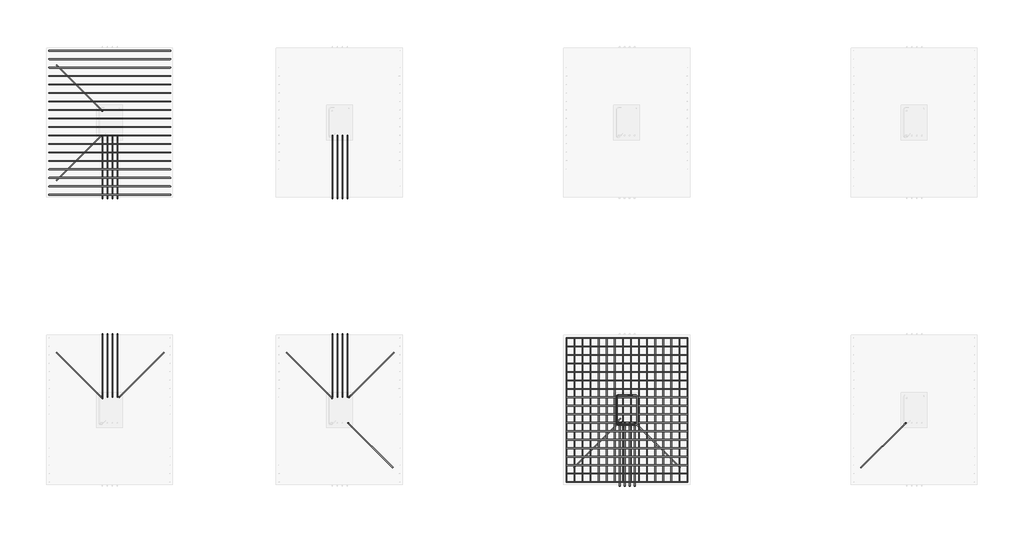
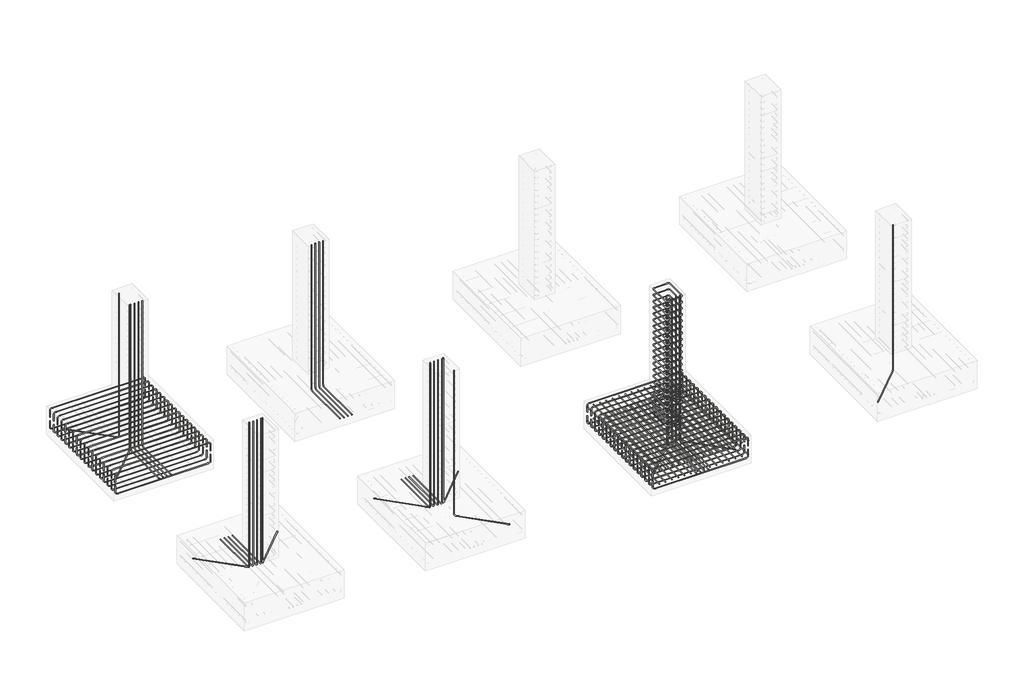
# One storey, part 4 of 33: 22 reinforcing bars.
"""IFC4 building model written with IfcOpenShell, lengths in millimetres."""

from ifc_helpers import new_model, si_unit, point, frame, origin, place, context, project, spatial, polyline, circle_curve, trimmed, segment, composite_curve, source, transform, mapped, element, save
from ifc_brep_helpers import swept_disk

model = new_model("IFC4")

# Units and contexts
model_context = context("Model", 3, world=origin())
ifc_project = project(units=[si_unit("LENGTHUNIT", "METRE", prefix="MILLI")], contexts=[model_context])

# Site, building, storey
site = spatial("IfcSite", under=ifc_project)
building = spatial("IfcBuilding", under=site)
storey = spatial("IfcBuildingStorey", under=building, Elevation=-3000.0)

# Reinforcing bars
placement = place(None, origin())
reinforcing_bar_shape = source(origin(), model_context, "Body", "SolidModel", [
    swept_disk(composite_curve([segment(polyline([(-5693.4642742, -7044.0608134, -3240.0), (-5693.4642742, -7044.0608134, -3092.7)]), True, "CONTINUOUS"), segment(trimmed(circle_curve(frame((-5647.1142742, -7044.0608134, -3092.7), z_axis=(0.0, 1.0, 0.0), x_axis=(-46.349999999999454, 0.0, 0.0)), 46.35), [point((-5693.4642742, -7044.0608134, -3092.7))], [point((-5647.1142742, -7044.0608134, -3046.35))], True, "CARTESIAN"), True, "CONTINUOUS"), segment(polyline([(-5647.1142742, -7044.0608134, -3046.35), (-3632.5142742, -7044.0608134, -3046.35)]), True, "CONTINUOUS"), segment(trimmed(circle_curve(frame((-3632.5142742, -7044.0608134, -3092.7), z_axis=(0.0, 1.0, 0.0), x_axis=(0.0, 0.0, 46.34999999999991)), 46.35), [point((-3632.5142742, -7044.0608134, -3046.35))], [point((-3586.1642742, -7044.0608134, -3092.7))], True, "CARTESIAN"), True, "CONTINUOUS"), segment(polyline([(-3586.1642742, -7044.0608134, -3092.7), (-3586.1642742, -7044.0608134, -3240.0)]), True, "CONTINUOUS")], self_intersect=False), 6.35),
])
element("IfcReinforcingBar", 1, at=placement, inside=storey, context=model_context, shape_type="MappedRepresentation", body=[
    mapped(reinforcing_bar_shape, transform((0.0, 0.0, 0.0), x_axis=(1.0, 0.0, 0.0), y_axis=(0.0, 1.0, 0.0), z_axis=(0.0, 0.0, 1.0))),
    mapped(reinforcing_bar_shape, transform((0.0, -147.4882353, 0.0), x_axis=(1.0, 0.0, 0.0), y_axis=(0.0, 1.0, 0.0), z_axis=(0.0, 0.0, 1.0))),
    mapped(reinforcing_bar_shape, transform((0.0, -294.9764706, 0.0), x_axis=(1.0, 0.0, 0.0), y_axis=(0.0, 1.0, 0.0), z_axis=(0.0, 0.0, 1.0))),
    mapped(reinforcing_bar_shape, transform((0.0, -442.4647059, 0.0), x_axis=(1.0, 0.0, 0.0), y_axis=(0.0, 1.0, 0.0), z_axis=(0.0, 0.0, 1.0))),
    mapped(reinforcing_bar_shape, transform((0.0, -589.9529412, 0.0), x_axis=(1.0, 0.0, 0.0), y_axis=(0.0, 1.0, 0.0), z_axis=(0.0, 0.0, 1.0))),
    mapped(reinforcing_bar_shape, transform((0.0, -737.4411765, 0.0), x_axis=(1.0, 0.0, 0.0), y_axis=(0.0, 1.0, 0.0), z_axis=(0.0, 0.0, 1.0))),
    mapped(reinforcing_bar_shape, transform((0.0, -884.9294118, 0.0), x_axis=(1.0, 0.0, 0.0), y_axis=(0.0, 1.0, 0.0), z_axis=(0.0, 0.0, 1.0))),
    mapped(reinforcing_bar_shape, transform((0.0, -1032.4176471, 0.0), x_axis=(1.0, 0.0, 0.0), y_axis=(0.0, 1.0, 0.0), z_axis=(0.0, 0.0, 1.0))),
    mapped(reinforcing_bar_shape, transform((0.0, -1179.9058824, 0.0), x_axis=(1.0, 0.0, 0.0), y_axis=(0.0, 1.0, 0.0), z_axis=(0.0, 0.0, 1.0))),
    mapped(reinforcing_bar_shape, transform((0.0, -1327.3941176, 0.0), x_axis=(1.0, 0.0, 0.0), y_axis=(0.0, 1.0, 0.0), z_axis=(0.0, 0.0, 1.0))),
    mapped(reinforcing_bar_shape, transform((0.0, -1474.8823529, 0.0), x_axis=(1.0, 0.0, 0.0), y_axis=(0.0, 1.0, 0.0), z_axis=(0.0, 0.0, 1.0))),
    mapped(reinforcing_bar_shape, transform((0.0, -1622.3705882, 0.0), x_axis=(1.0, 0.0, 0.0), y_axis=(0.0, 1.0, 0.0), z_axis=(0.0, 0.0, 1.0))),
    mapped(reinforcing_bar_shape, transform((0.0, -1769.8588235, 0.0), x_axis=(1.0, 0.0, 0.0), y_axis=(0.0, 1.0, 0.0), z_axis=(0.0, 0.0, 1.0))),
    mapped(reinforcing_bar_shape, transform((0.0, -1917.3470588, 0.0), x_axis=(1.0, 0.0, 0.0), y_axis=(0.0, 1.0, 0.0), z_axis=(0.0, 0.0, 1.0))),
    mapped(reinforcing_bar_shape, transform((0.0, -2064.8352941, 0.0), x_axis=(1.0, 0.0, 0.0), y_axis=(0.0, 1.0, 0.0), z_axis=(0.0, 0.0, 1.0))),
    mapped(reinforcing_bar_shape, transform((0.0, -2212.3235294, 0.0), x_axis=(1.0, 0.0, 0.0), y_axis=(0.0, 1.0, 0.0), z_axis=(0.0, 0.0, 1.0))),
    mapped(reinforcing_bar_shape, transform((0.0, -2359.8117647, 0.0), x_axis=(1.0, 0.0, 0.0), y_axis=(0.0, 1.0, 0.0), z_axis=(0.0, 0.0, 1.0))),
    mapped(reinforcing_bar_shape, transform((0.0, -2507.3, 0.0), x_axis=(1.0, 0.0, 0.0), y_axis=(0.0, 1.0, 0.0), z_axis=(0.0, 0.0, 1.0))),
])
reinforcing_bar_2_shape = source(origin(), model_context, "Body", "SolidModel", [
    swept_disk(composite_curve([segment(polyline([(-3586.1642742, -7044.0608134, -3330.080452), (-3586.1642742, -7044.0608134, -3477.380452)]), True, "CONTINUOUS"), segment(trimmed(circle_curve(frame((-3632.5142742, -7044.0608134, -3477.380452), z_axis=(0.0, 1.0, 0.0), x_axis=(46.34999999999991, 0.0, 0.0)), 46.35), [point((-3586.1642742, -7044.0608134, -3477.380452))], [point((-3632.5142742, -7044.0608134, -3523.730452))], True, "CARTESIAN"), True, "CONTINUOUS"), segment(polyline([(-3632.5142742, -7044.0608134, -3523.730452), (-5647.1142742, -7044.0608134, -3523.730452)]), True, "CONTINUOUS"), segment(trimmed(circle_curve(frame((-5647.1142742, -7044.0608134, -3477.380452), z_axis=(0.0, 1.0, 0.0), x_axis=(0.0, 0.0, -46.34999999999991)), 46.35), [point((-5647.1142742, -7044.0608134, -3523.730452))], [point((-5693.4642742, -7044.0608134, -3477.380452))], True, "CARTESIAN"), True, "CONTINUOUS"), segment(polyline([(-5693.4642742, -7044.0608134, -3477.380452), (-5693.4642742, -7044.0608134, -3330.080452)]), True, "CONTINUOUS")], self_intersect=False), 6.35),
])
element("IfcReinforcingBar", 2, at=placement, inside=storey, context=model_context, shape_type="MappedRepresentation", body=[
    mapped(reinforcing_bar_2_shape, transform((0.0, 0.0, 0.0), x_axis=(1.0, 0.0, 0.0), y_axis=(0.0, 1.0, 0.0), z_axis=(0.0, 0.0, 1.0))),
    mapped(reinforcing_bar_2_shape, transform((0.0, -147.4882353, 0.0), x_axis=(1.0, 0.0, 0.0), y_axis=(0.0, 1.0, 0.0), z_axis=(0.0, 0.0, 1.0))),
    mapped(reinforcing_bar_2_shape, transform((0.0, -294.9764706, 0.0), x_axis=(1.0, 0.0, 0.0), y_axis=(0.0, 1.0, 0.0), z_axis=(0.0, 0.0, 1.0))),
    mapped(reinforcing_bar_2_shape, transform((0.0, -442.4647059, 0.0), x_axis=(1.0, 0.0, 0.0), y_axis=(0.0, 1.0, 0.0), z_axis=(0.0, 0.0, 1.0))),
    mapped(reinforcing_bar_2_shape, transform((0.0, -589.9529412, 0.0), x_axis=(1.0, 0.0, 0.0), y_axis=(0.0, 1.0, 0.0), z_axis=(0.0, 0.0, 1.0))),
    mapped(reinforcing_bar_2_shape, transform((0.0, -737.4411765, 0.0), x_axis=(1.0, 0.0, 0.0), y_axis=(0.0, 1.0, 0.0), z_axis=(0.0, 0.0, 1.0))),
    mapped(reinforcing_bar_2_shape, transform((0.0, -884.9294118, 0.0), x_axis=(1.0, 0.0, 0.0), y_axis=(0.0, 1.0, 0.0), z_axis=(0.0, 0.0, 1.0))),
    mapped(reinforcing_bar_2_shape, transform((0.0, -1032.4176471, 0.0), x_axis=(1.0, 0.0, 0.0), y_axis=(0.0, 1.0, 0.0), z_axis=(0.0, 0.0, 1.0))),
    mapped(reinforcing_bar_2_shape, transform((0.0, -1179.9058824, 0.0), x_axis=(1.0, 0.0, 0.0), y_axis=(0.0, 1.0, 0.0), z_axis=(0.0, 0.0, 1.0))),
    mapped(reinforcing_bar_2_shape, transform((0.0, -1327.3941176, 0.0), x_axis=(1.0, 0.0, 0.0), y_axis=(0.0, 1.0, 0.0), z_axis=(0.0, 0.0, 1.0))),
    mapped(reinforcing_bar_2_shape, transform((0.0, -1474.8823529, 0.0), x_axis=(1.0, 0.0, 0.0), y_axis=(0.0, 1.0, 0.0), z_axis=(0.0, 0.0, 1.0))),
    mapped(reinforcing_bar_2_shape, transform((0.0, -1622.3705882, 0.0), x_axis=(1.0, 0.0, 0.0), y_axis=(0.0, 1.0, 0.0), z_axis=(0.0, 0.0, 1.0))),
    mapped(reinforcing_bar_2_shape, transform((0.0, -1769.8588235, 0.0), x_axis=(1.0, 0.0, 0.0), y_axis=(0.0, 1.0, 0.0), z_axis=(0.0, 0.0, 1.0))),
    mapped(reinforcing_bar_2_shape, transform((0.0, -1917.3470588, 0.0), x_axis=(1.0, 0.0, 0.0), y_axis=(0.0, 1.0, 0.0), z_axis=(0.0, 0.0, 1.0))),
    mapped(reinforcing_bar_2_shape, transform((0.0, -2064.8352941, 0.0), x_axis=(1.0, 0.0, 0.0), y_axis=(0.0, 1.0, 0.0), z_axis=(0.0, 0.0, 1.0))),
    mapped(reinforcing_bar_2_shape, transform((0.0, -2212.3235294, 0.0), x_axis=(1.0, 0.0, 0.0), y_axis=(0.0, 1.0, 0.0), z_axis=(0.0, 0.0, 1.0))),
    mapped(reinforcing_bar_2_shape, transform((0.0, -2359.8117647, 0.0), x_axis=(1.0, 0.0, 0.0), y_axis=(0.0, 1.0, 0.0), z_axis=(0.0, 0.0, 1.0))),
    mapped(reinforcing_bar_2_shape, transform((0.0, -2507.3, 0.0), x_axis=(1.0, 0.0, 0.0), y_axis=(0.0, 1.0, 0.0), z_axis=(0.0, 0.0, 1.0))),
])
reinforcing_bar_3_shape = source(origin(), model_context, "Body", "SolidModel", [
    swept_disk(composite_curve([segment(polyline([(-3586.1642742, -9557.7108134, -3447.8614173), (-3586.1642742, -7037.7108134, -3447.8614173)]), True, "CONTINUOUS")], self_intersect=False), 6.35),
])
element("IfcReinforcingBar", 3, at=placement, inside=storey, context=model_context, shape_type="MappedRepresentation", body=[
    mapped(reinforcing_bar_3_shape, transform((0.0, 0.0, 0.0), x_axis=(1.0, 0.0, 0.0), y_axis=(0.0, 1.0, 0.0), z_axis=(0.0, 0.0, 1.0))),
    mapped(reinforcing_bar_3_shape, transform((-140.4866667, 0.0, 0.0), x_axis=(1.0, 0.0, 0.0), y_axis=(0.0, 1.0, 0.0), z_axis=(0.0, 0.0, 1.0))),
    mapped(reinforcing_bar_3_shape, transform((-280.9733333, 0.0, 0.0), x_axis=(1.0, 0.0, 0.0), y_axis=(0.0, 1.0, 0.0), z_axis=(0.0, 0.0, 1.0))),
    mapped(reinforcing_bar_3_shape, transform((-421.46, 0.0, 0.0), x_axis=(1.0, 0.0, 0.0), y_axis=(0.0, 1.0, 0.0), z_axis=(0.0, 0.0, 1.0))),
    mapped(reinforcing_bar_3_shape, transform((-561.9466667, 0.0, 0.0), x_axis=(1.0, 0.0, 0.0), y_axis=(0.0, 1.0, 0.0), z_axis=(0.0, 0.0, 1.0))),
    mapped(reinforcing_bar_3_shape, transform((-702.4333333, 0.0, 0.0), x_axis=(1.0, 0.0, 0.0), y_axis=(0.0, 1.0, 0.0), z_axis=(0.0, 0.0, 1.0))),
    mapped(reinforcing_bar_3_shape, transform((-842.92, 0.0, 0.0), x_axis=(1.0, 0.0, 0.0), y_axis=(0.0, 1.0, 0.0), z_axis=(0.0, 0.0, 1.0))),
    mapped(reinforcing_bar_3_shape, transform((-983.4066667, 0.0, 0.0), x_axis=(1.0, 0.0, 0.0), y_axis=(0.0, 1.0, 0.0), z_axis=(0.0, 0.0, 1.0))),
    mapped(reinforcing_bar_3_shape, transform((-1123.8933333, 0.0, 0.0), x_axis=(1.0, 0.0, 0.0), y_axis=(0.0, 1.0, 0.0), z_axis=(0.0, 0.0, 1.0))),
    mapped(reinforcing_bar_3_shape, transform((-1264.38, 0.0, 0.0), x_axis=(1.0, 0.0, 0.0), y_axis=(0.0, 1.0, 0.0), z_axis=(0.0, 0.0, 1.0))),
    mapped(reinforcing_bar_3_shape, transform((-1404.8666667, 0.0, 0.0), x_axis=(1.0, 0.0, 0.0), y_axis=(0.0, 1.0, 0.0), z_axis=(0.0, 0.0, 1.0))),
    mapped(reinforcing_bar_3_shape, transform((-1545.3533333, 0.0, 0.0), x_axis=(1.0, 0.0, 0.0), y_axis=(0.0, 1.0, 0.0), z_axis=(0.0, 0.0, 1.0))),
    mapped(reinforcing_bar_3_shape, transform((-1685.84, 0.0, 0.0), x_axis=(1.0, 0.0, 0.0), y_axis=(0.0, 1.0, 0.0), z_axis=(0.0, 0.0, 1.0))),
    mapped(reinforcing_bar_3_shape, transform((-1826.3266667, 0.0, 0.0), x_axis=(1.0, 0.0, 0.0), y_axis=(0.0, 1.0, 0.0), z_axis=(0.0, 0.0, 1.0))),
    mapped(reinforcing_bar_3_shape, transform((-1966.8133333, 0.0, 0.0), x_axis=(1.0, 0.0, 0.0), y_axis=(0.0, 1.0, 0.0), z_axis=(0.0, 0.0, 1.0))),
    mapped(reinforcing_bar_3_shape, transform((-2107.3, 0.0, 0.0), x_axis=(1.0, 0.0, 0.0), y_axis=(0.0, 1.0, 0.0), z_axis=(0.0, 0.0, 1.0))),
])
reinforcing_bar_4_shape = source(origin(), model_context, "Body", "SolidModel", [
    swept_disk(composite_curve([segment(polyline([(-5693.4642742, -9557.7108134, -3122.7084113), (-5693.4642742, -7037.7108134, -3122.7084113)]), True, "CONTINUOUS")], self_intersect=False), 6.35),
])
element("IfcReinforcingBar", 4, at=placement, inside=storey, context=model_context, shape_type="MappedRepresentation", body=[
    mapped(reinforcing_bar_4_shape, transform((0.0, 0.0, 0.0), x_axis=(1.0, 0.0, 0.0), y_axis=(0.0, 1.0, 0.0), z_axis=(0.0, 0.0, 1.0))),
    mapped(reinforcing_bar_4_shape, transform((140.4866667, 0.0, 0.0), x_axis=(1.0, 0.0, 0.0), y_axis=(0.0, 1.0, 0.0), z_axis=(0.0, 0.0, 1.0))),
    mapped(reinforcing_bar_4_shape, transform((280.9733333, 0.0, 0.0), x_axis=(1.0, 0.0, 0.0), y_axis=(0.0, 1.0, 0.0), z_axis=(0.0, 0.0, 1.0))),
    mapped(reinforcing_bar_4_shape, transform((421.46, 0.0, 0.0), x_axis=(1.0, 0.0, 0.0), y_axis=(0.0, 1.0, 0.0), z_axis=(0.0, 0.0, 1.0))),
    mapped(reinforcing_bar_4_shape, transform((561.9466667, 0.0, 0.0), x_axis=(1.0, 0.0, 0.0), y_axis=(0.0, 1.0, 0.0), z_axis=(0.0, 0.0, 1.0))),
    mapped(reinforcing_bar_4_shape, transform((702.4333333, 0.0, 0.0), x_axis=(1.0, 0.0, 0.0), y_axis=(0.0, 1.0, 0.0), z_axis=(0.0, 0.0, 1.0))),
    mapped(reinforcing_bar_4_shape, transform((842.92, 0.0, 0.0), x_axis=(1.0, 0.0, 0.0), y_axis=(0.0, 1.0, 0.0), z_axis=(0.0, 0.0, 1.0))),
    mapped(reinforcing_bar_4_shape, transform((983.4066667, 0.0, 0.0), x_axis=(1.0, 0.0, 0.0), y_axis=(0.0, 1.0, 0.0), z_axis=(0.0, 0.0, 1.0))),
    mapped(reinforcing_bar_4_shape, transform((1123.8933333, 0.0, 0.0), x_axis=(1.0, 0.0, 0.0), y_axis=(0.0, 1.0, 0.0), z_axis=(0.0, 0.0, 1.0))),
    mapped(reinforcing_bar_4_shape, transform((1264.38, 0.0, 0.0), x_axis=(1.0, 0.0, 0.0), y_axis=(0.0, 1.0, 0.0), z_axis=(0.0, 0.0, 1.0))),
    mapped(reinforcing_bar_4_shape, transform((1404.8666667, 0.0, 0.0), x_axis=(1.0, 0.0, 0.0), y_axis=(0.0, 1.0, 0.0), z_axis=(0.0, 0.0, 1.0))),
    mapped(reinforcing_bar_4_shape, transform((1545.3533333, 0.0, 0.0), x_axis=(1.0, 0.0, 0.0), y_axis=(0.0, 1.0, 0.0), z_axis=(0.0, 0.0, 1.0))),
    mapped(reinforcing_bar_4_shape, transform((1685.84, 0.0, 0.0), x_axis=(1.0, 0.0, 0.0), y_axis=(0.0, 1.0, 0.0), z_axis=(0.0, 0.0, 1.0))),
    mapped(reinforcing_bar_4_shape, transform((1826.3266667, 0.0, 0.0), x_axis=(1.0, 0.0, 0.0), y_axis=(0.0, 1.0, 0.0), z_axis=(0.0, 0.0, 1.0))),
    mapped(reinforcing_bar_4_shape, transform((1966.8133333, 0.0, 0.0), x_axis=(1.0, 0.0, 0.0), y_axis=(0.0, 1.0, 0.0), z_axis=(0.0, 0.0, 1.0))),
    mapped(reinforcing_bar_4_shape, transform((2107.3, 0.0, 0.0), x_axis=(1.0, 0.0, 0.0), y_axis=(0.0, 1.0, 0.0), z_axis=(0.0, 0.0, 1.0))),
])
reinforcing_bar_5_shape = source(origin(), model_context, "Body", "SolidModel", [
    swept_disk(composite_curve([segment(polyline([(-14693.4642742, -2044.0608134, -3240.0), (-14693.4642742, -2044.0608134, -3092.7)]), True, "CONTINUOUS"), segment(trimmed(circle_curve(frame((-14647.1142742, -2044.0608134, -3092.7), z_axis=(0.0, 1.0, 0.0), x_axis=(-46.350000000000364, 0.0, 0.0)), 46.35), [point((-14693.4642742, -2044.0608134, -3092.7))], [point((-14647.1142742, -2044.0608134, -3046.35))], True, "CARTESIAN"), True, "CONTINUOUS"), segment(polyline([(-14647.1142742, -2044.0608134, -3046.35), (-12632.5142742, -2044.0608134, -3046.35)]), True, "CONTINUOUS"), segment(trimmed(circle_curve(frame((-12632.5142742, -2044.0608134, -3092.7), z_axis=(0.0, 1.0, 0.0), x_axis=(0.0, 0.0, 46.34999999999991)), 46.35), [point((-12632.5142742, -2044.0608134, -3046.35))], [point((-12586.1642742, -2044.0608134, -3092.7))], True, "CARTESIAN"), True, "CONTINUOUS"), segment(polyline([(-12586.1642742, -2044.0608134, -3092.7), (-12586.1642742, -2044.0608134, -3240.0)]), True, "CONTINUOUS")], self_intersect=False), 6.35),
])
element("IfcReinforcingBar", 5, at=placement, inside=storey, context=model_context, shape_type="MappedRepresentation", body=[
    mapped(reinforcing_bar_5_shape, transform((0.0, 0.0, 0.0), x_axis=(1.0, 0.0, 0.0), y_axis=(0.0, 1.0, 0.0), z_axis=(0.0, 0.0, 1.0))),
    mapped(reinforcing_bar_5_shape, transform((0.0, -147.4882353, 0.0), x_axis=(1.0, 0.0, 0.0), y_axis=(0.0, 1.0, 0.0), z_axis=(0.0, 0.0, 1.0))),
    mapped(reinforcing_bar_5_shape, transform((0.0, -294.9764706, 0.0), x_axis=(1.0, 0.0, 0.0), y_axis=(0.0, 1.0, 0.0), z_axis=(0.0, 0.0, 1.0))),
    mapped(reinforcing_bar_5_shape, transform((0.0, -442.4647059, 0.0), x_axis=(1.0, 0.0, 0.0), y_axis=(0.0, 1.0, 0.0), z_axis=(0.0, 0.0, 1.0))),
    mapped(reinforcing_bar_5_shape, transform((0.0, -589.9529412, 0.0), x_axis=(1.0, 0.0, 0.0), y_axis=(0.0, 1.0, 0.0), z_axis=(0.0, 0.0, 1.0))),
    mapped(reinforcing_bar_5_shape, transform((0.0, -737.4411765, 0.0), x_axis=(1.0, 0.0, 0.0), y_axis=(0.0, 1.0, 0.0), z_axis=(0.0, 0.0, 1.0))),
    mapped(reinforcing_bar_5_shape, transform((0.0, -884.9294118, 0.0), x_axis=(1.0, 0.0, 0.0), y_axis=(0.0, 1.0, 0.0), z_axis=(0.0, 0.0, 1.0))),
    mapped(reinforcing_bar_5_shape, transform((0.0, -1032.4176471, 0.0), x_axis=(1.0, 0.0, 0.0), y_axis=(0.0, 1.0, 0.0), z_axis=(0.0, 0.0, 1.0))),
    mapped(reinforcing_bar_5_shape, transform((0.0, -1179.9058824, 0.0), x_axis=(1.0, 0.0, 0.0), y_axis=(0.0, 1.0, 0.0), z_axis=(0.0, 0.0, 1.0))),
    mapped(reinforcing_bar_5_shape, transform((0.0, -1327.3941176, 0.0), x_axis=(1.0, 0.0, 0.0), y_axis=(0.0, 1.0, 0.0), z_axis=(0.0, 0.0, 1.0))),
    mapped(reinforcing_bar_5_shape, transform((0.0, -1474.8823529, 0.0), x_axis=(1.0, 0.0, 0.0), y_axis=(0.0, 1.0, 0.0), z_axis=(0.0, 0.0, 1.0))),
    mapped(reinforcing_bar_5_shape, transform((0.0, -1622.3705882, 0.0), x_axis=(1.0, 0.0, 0.0), y_axis=(0.0, 1.0, 0.0), z_axis=(0.0, 0.0, 1.0))),
    mapped(reinforcing_bar_5_shape, transform((0.0, -1769.8588235, 0.0), x_axis=(1.0, 0.0, 0.0), y_axis=(0.0, 1.0, 0.0), z_axis=(0.0, 0.0, 1.0))),
    mapped(reinforcing_bar_5_shape, transform((0.0, -1917.3470588, 0.0), x_axis=(1.0, 0.0, 0.0), y_axis=(0.0, 1.0, 0.0), z_axis=(0.0, 0.0, 1.0))),
    mapped(reinforcing_bar_5_shape, transform((0.0, -2064.8352941, 0.0), x_axis=(1.0, 0.0, 0.0), y_axis=(0.0, 1.0, 0.0), z_axis=(0.0, 0.0, 1.0))),
    mapped(reinforcing_bar_5_shape, transform((0.0, -2212.3235294, 0.0), x_axis=(1.0, 0.0, 0.0), y_axis=(0.0, 1.0, 0.0), z_axis=(0.0, 0.0, 1.0))),
    mapped(reinforcing_bar_5_shape, transform((0.0, -2359.8117647, 0.0), x_axis=(1.0, 0.0, 0.0), y_axis=(0.0, 1.0, 0.0), z_axis=(0.0, 0.0, 1.0))),
    mapped(reinforcing_bar_5_shape, transform((0.0, -2507.3, 0.0), x_axis=(1.0, 0.0, 0.0), y_axis=(0.0, 1.0, 0.0), z_axis=(0.0, 0.0, 1.0))),
])
reinforcing_bar_6_shape = source(origin(), model_context, "Body", "SolidModel", [
    swept_disk(composite_curve([segment(polyline([(-12586.1642742, -2044.0608134, -3330.080452), (-12586.1642742, -2044.0608134, -3477.380452)]), True, "CONTINUOUS"), segment(trimmed(circle_curve(frame((-12632.5142742, -2044.0608134, -3477.380452), z_axis=(0.0, 1.0, 0.0), x_axis=(46.350000000000364, 0.0, 0.0)), 46.35), [point((-12586.1642742, -2044.0608134, -3477.380452))], [point((-12632.5142742, -2044.0608134, -3523.730452))], True, "CARTESIAN"), True, "CONTINUOUS"), segment(polyline([(-12632.5142742, -2044.0608134, -3523.730452), (-14647.1142742, -2044.0608134, -3523.730452)]), True, "CONTINUOUS"), segment(trimmed(circle_curve(frame((-14647.1142742, -2044.0608134, -3477.380452), z_axis=(0.0, 1.0, 0.0), x_axis=(0.0, 0.0, -46.34999999999991)), 46.35), [point((-14647.1142742, -2044.0608134, -3523.730452))], [point((-14693.4642742, -2044.0608134, -3477.380452))], True, "CARTESIAN"), True, "CONTINUOUS"), segment(polyline([(-14693.4642742, -2044.0608134, -3477.380452), (-14693.4642742, -2044.0608134, -3330.080452)]), True, "CONTINUOUS")], self_intersect=False), 6.35),
])
element("IfcReinforcingBar", 6, at=placement, inside=storey, context=model_context, shape_type="MappedRepresentation", body=[
    mapped(reinforcing_bar_6_shape, transform((0.0, 0.0, 0.0), x_axis=(1.0, 0.0, 0.0), y_axis=(0.0, 1.0, 0.0), z_axis=(0.0, 0.0, 1.0))),
    mapped(reinforcing_bar_6_shape, transform((0.0, -147.4882353, 0.0), x_axis=(1.0, 0.0, 0.0), y_axis=(0.0, 1.0, 0.0), z_axis=(0.0, 0.0, 1.0))),
    mapped(reinforcing_bar_6_shape, transform((0.0, -294.9764706, 0.0), x_axis=(1.0, 0.0, 0.0), y_axis=(0.0, 1.0, 0.0), z_axis=(0.0, 0.0, 1.0))),
    mapped(reinforcing_bar_6_shape, transform((0.0, -442.4647059, 0.0), x_axis=(1.0, 0.0, 0.0), y_axis=(0.0, 1.0, 0.0), z_axis=(0.0, 0.0, 1.0))),
    mapped(reinforcing_bar_6_shape, transform((0.0, -589.9529412, 0.0), x_axis=(1.0, 0.0, 0.0), y_axis=(0.0, 1.0, 0.0), z_axis=(0.0, 0.0, 1.0))),
    mapped(reinforcing_bar_6_shape, transform((0.0, -737.4411765, 0.0), x_axis=(1.0, 0.0, 0.0), y_axis=(0.0, 1.0, 0.0), z_axis=(0.0, 0.0, 1.0))),
    mapped(reinforcing_bar_6_shape, transform((0.0, -884.9294118, 0.0), x_axis=(1.0, 0.0, 0.0), y_axis=(0.0, 1.0, 0.0), z_axis=(0.0, 0.0, 1.0))),
    mapped(reinforcing_bar_6_shape, transform((0.0, -1032.4176471, 0.0), x_axis=(1.0, 0.0, 0.0), y_axis=(0.0, 1.0, 0.0), z_axis=(0.0, 0.0, 1.0))),
    mapped(reinforcing_bar_6_shape, transform((0.0, -1179.9058824, 0.0), x_axis=(1.0, 0.0, 0.0), y_axis=(0.0, 1.0, 0.0), z_axis=(0.0, 0.0, 1.0))),
    mapped(reinforcing_bar_6_shape, transform((0.0, -1327.3941176, 0.0), x_axis=(1.0, 0.0, 0.0), y_axis=(0.0, 1.0, 0.0), z_axis=(0.0, 0.0, 1.0))),
    mapped(reinforcing_bar_6_shape, transform((0.0, -1474.8823529, 0.0), x_axis=(1.0, 0.0, 0.0), y_axis=(0.0, 1.0, 0.0), z_axis=(0.0, 0.0, 1.0))),
    mapped(reinforcing_bar_6_shape, transform((0.0, -1622.3705882, 0.0), x_axis=(1.0, 0.0, 0.0), y_axis=(0.0, 1.0, 0.0), z_axis=(0.0, 0.0, 1.0))),
    mapped(reinforcing_bar_6_shape, transform((0.0, -1769.8588235, 0.0), x_axis=(1.0, 0.0, 0.0), y_axis=(0.0, 1.0, 0.0), z_axis=(0.0, 0.0, 1.0))),
    mapped(reinforcing_bar_6_shape, transform((0.0, -1917.3470588, 0.0), x_axis=(1.0, 0.0, 0.0), y_axis=(0.0, 1.0, 0.0), z_axis=(0.0, 0.0, 1.0))),
    mapped(reinforcing_bar_6_shape, transform((0.0, -2064.8352941, 0.0), x_axis=(1.0, 0.0, 0.0), y_axis=(0.0, 1.0, 0.0), z_axis=(0.0, 0.0, 1.0))),
    mapped(reinforcing_bar_6_shape, transform((0.0, -2212.3235294, 0.0), x_axis=(1.0, 0.0, 0.0), y_axis=(0.0, 1.0, 0.0), z_axis=(0.0, 0.0, 1.0))),
    mapped(reinforcing_bar_6_shape, transform((0.0, -2359.8117647, 0.0), x_axis=(1.0, 0.0, 0.0), y_axis=(0.0, 1.0, 0.0), z_axis=(0.0, 0.0, 1.0))),
    mapped(reinforcing_bar_6_shape, transform((0.0, -2507.3, 0.0), x_axis=(1.0, 0.0, 0.0), y_axis=(0.0, 1.0, 0.0), z_axis=(0.0, 0.0, 1.0))),
])
element("IfcReinforcingBar", 7, at=placement, inside=storey, context=model_context, shape_type="SolidModel", body=[
    swept_disk(composite_curve([segment(polyline([(-13786.7956786, -3521.6339414, -40.0), (-13786.7956786, -3521.6339414, -3393.65)]), True, "CONTINUOUS"), segment(trimmed(circle_curve(frame((-13819.5700779, -3554.4083407, -3393.65), z_axis=(-0.7071067811865446, 0.7071067811865505, 0.0), x_axis=(32.77439930000037, 32.774399299999914, 0.0)), 46.35), [point((-13786.7956786, -3521.6339414, -3393.65))], [point((-13819.5700779, -3554.4083407, -3440.0))], True, "CARTESIAN"), True, "CONTINUOUS"), segment(polyline([(-13819.5700779, -3554.4083407, -3440.0), (-14564.6131379, -4299.4514007, -3440.0)]), True, "CONTINUOUS")], self_intersect=False), 6.35),
])
element("IfcReinforcingBar", 8, at=placement, inside=storey, context=model_context, shape_type="SolidModel", body=[
    swept_disk(composite_curve([segment(polyline([(-13768.8975726, -3091.6857913, -40.0), (-13768.8975726, -3091.6857913, -3361.434517)]), True, "CONTINUOUS"), segment(trimmed(circle_curve(frame((-13801.6719719, -3058.911392, -3361.434517), z_axis=(0.7071067811865539, 0.7071067811865411, 0.0), x_axis=(32.77439929999855, -32.774399299999914, 0.0)), 46.35), [point((-13768.8975726, -3091.6857913, -3361.434517))], [point((-13801.6719719, -3058.911392, -3407.784517))], True, "CARTESIAN"), True, "CONTINUOUS"), segment(polyline([(-13801.6719719, -3058.911392, -3407.784517), (-14564.6131379, -2295.970226, -3407.784517)]), True, "CONTINUOUS")], self_intersect=False), 6.35),
])
reinforcing_bar_7_shape = source(origin(), model_context, "Body", "SolidModel", [
    swept_disk(composite_curve([segment(polyline([(-13763.8841678, -3523.4938134, -40.0), (-13763.8841678, -3523.4938134, -3393.65)]), True, "CONTINUOUS"), segment(trimmed(circle_curve(frame((-13763.8841678, -3569.8438134, -3393.65), z_axis=(-1.0, 0.0, 0.0), x_axis=(0.0, 46.34999999999991, 0.0)), 46.35), [point((-13763.8841678, -3523.4938134, -3393.65))], [point((-13763.8841678, -3569.8438134, -3440.0))], True, "CARTESIAN"), True, "CONTINUOUS"), segment(polyline([(-13763.8841678, -3569.8438134, -3440.0), (-13763.8841678, -4623.4938134, -3440.0)]), True, "CONTINUOUS")], self_intersect=False), 6.35),
])
element("IfcReinforcingBar", 9, at=placement, inside=storey, context=model_context, shape_type="MappedRepresentation", body=[
    mapped(reinforcing_bar_7_shape, transform((0.0, 0.0, 0.0), x_axis=(1.0, 0.0, 0.0), y_axis=(0.0, 1.0, 0.0), z_axis=(0.0, 0.0, 1.0))),
    mapped(reinforcing_bar_7_shape, transform((86.8979716, 0.0, 0.0), x_axis=(1.0, 0.0, 0.0), y_axis=(0.0, 1.0, 0.0), z_axis=(0.0, 0.0, 1.0))),
    mapped(reinforcing_bar_7_shape, transform((173.7959432, 0.0, 0.0), x_axis=(1.0, 0.0, 0.0), y_axis=(0.0, 1.0, 0.0), z_axis=(0.0, 0.0, 1.0))),
    mapped(reinforcing_bar_7_shape, transform((260.6939148, 0.0, 0.0), x_axis=(1.0, 0.0, 0.0), y_axis=(0.0, 1.0, 0.0), z_axis=(0.0, 0.0, 1.0))),
])
element("IfcReinforcingBar", 10, at=placement, inside=storey, context=model_context, shape_type="SolidModel", body=[
    swept_disk(composite_curve([segment(polyline([(-13768.8975726, -8091.6857913, -40.0), (-13768.8975726, -8091.6857913, -3361.434517)]), True, "CONTINUOUS"), segment(trimmed(circle_curve(frame((-13801.6719719, -8058.911392, -3361.434517), z_axis=(0.7071067811865539, 0.7071067811865411, 0.0), x_axis=(32.77439929999855, -32.77439930000037, 0.0)), 46.35), [point((-13768.8975726, -8091.6857913, -3361.434517))], [point((-13801.6719719, -8058.911392, -3407.784517))], True, "CARTESIAN"), True, "CONTINUOUS"), segment(polyline([(-13801.6719719, -8058.911392, -3407.784517), (-14564.6131379, -7295.970226, -3407.784517)]), True, "CONTINUOUS")], self_intersect=False), 6.35),
])
element("IfcReinforcingBar", 11, at=placement, inside=storey, context=model_context, shape_type="SolidModel", body=[
    swept_disk(composite_curve([segment(polyline([(-13474.2315783, -8073.7876853, -30.2564663), (-13474.2315783, -8073.7876853, -3383.9064663)]), True, "CONTINUOUS"), segment(trimmed(circle_curve(frame((-13441.457179, -8041.013286, -3383.9064663), z_axis=(0.7071067811865493, -0.7071067811865459, 0.0), x_axis=(-32.77439929999855, -32.77439929999946, 0.0)), 46.35), [point((-13474.2315783, -8073.7876853, -3383.9064663))], [point((-13441.457179, -8041.013286, -3430.2564663))], True, "CARTESIAN"), True, "CONTINUOUS"), segment(polyline([(-13441.457179, -8041.013286, -3430.2564663), (-12696.414119, -7295.970226, -3430.2564663)]), True, "CONTINUOUS")], self_intersect=False), 6.35),
])
reinforcing_bar_8_shape = source(origin(), model_context, "Body", "SolidModel", [
    swept_disk(composite_curve([segment(polyline([(-13763.8841678, -8071.9278134, -40.0), (-13763.8841678, -8071.9278134, -3393.65)]), True, "CONTINUOUS"), segment(trimmed(circle_curve(frame((-13763.8841678, -8025.5778134, -3393.65), z_axis=(1.0, 0.0, 0.0), x_axis=(0.0, -46.349999999999454, 0.0)), 46.35), [point((-13763.8841678, -8071.9278134, -3393.65))], [point((-13763.8841678, -8025.5778134, -3440.0))], True, "CARTESIAN"), True, "CONTINUOUS"), segment(polyline([(-13763.8841678, -8025.5778134, -3440.0), (-13763.8841678, -6971.9278134, -3440.0)]), True, "CONTINUOUS")], self_intersect=False), 6.35),
])
element("IfcReinforcingBar", 12, at=placement, inside=storey, context=model_context, shape_type="MappedRepresentation", body=[
    mapped(reinforcing_bar_8_shape, transform((0.0, 0.0, 0.0), x_axis=(1.0, 0.0, 0.0), y_axis=(0.0, 1.0, 0.0), z_axis=(0.0, 0.0, 1.0))),
    mapped(reinforcing_bar_8_shape, transform((86.8979716, 0.0, 0.0), x_axis=(1.0, 0.0, 0.0), y_axis=(0.0, 1.0, 0.0), z_axis=(0.0, 0.0, 1.0))),
    mapped(reinforcing_bar_8_shape, transform((173.7959432, 0.0, 0.0), x_axis=(1.0, 0.0, 0.0), y_axis=(0.0, 1.0, 0.0), z_axis=(0.0, 0.0, 1.0))),
    mapped(reinforcing_bar_8_shape, transform((260.6939148, 0.0, 0.0), x_axis=(1.0, 0.0, 0.0), y_axis=(0.0, 1.0, 0.0), z_axis=(0.0, 0.0, 1.0))),
])
element("IfcReinforcingBar", 13, at=placement, inside=storey, context=model_context, shape_type="SolidModel", body=[
    swept_disk(composite_curve([segment(polyline([(-9768.8975726, -8091.6857913, -40.0), (-9768.8975726, -8091.6857913, -3361.434517)]), True, "CONTINUOUS"), segment(trimmed(circle_curve(frame((-9801.6719719, -8058.911392, -3361.434517), z_axis=(0.7071067811865539, 0.7071067811865411, 0.0), x_axis=(32.77439929999855, -32.77439930000037, 0.0)), 46.35), [point((-9768.8975726, -8091.6857913, -3361.434517))], [point((-9801.6719719, -8058.911392, -3407.784517))], True, "CARTESIAN"), True, "CONTINUOUS"), segment(polyline([(-9801.6719719, -8058.911392, -3407.784517), (-10564.6131379, -7295.970226, -3407.784517)]), True, "CONTINUOUS")], self_intersect=False), 6.35),
])
element("IfcReinforcingBar", 14, at=placement, inside=storey, context=model_context, shape_type="SolidModel", body=[
    swept_disk(composite_curve([segment(polyline([(-9492.8328699, -8521.6339414, -40.0), (-9492.8328699, -8521.6339414, -3393.65)]), True, "CONTINUOUS"), segment(trimmed(circle_curve(frame((-9460.0584706, -8554.4083407, -3393.65), z_axis=(-0.7071067811865493, -0.7071067811865459, 0.0), x_axis=(-32.77439929999855, 32.77439930000037, 0.0)), 46.35), [point((-9492.8328699, -8521.6339414, -3393.65))], [point((-9460.0584706, -8554.4083407, -3440.0))], True, "CARTESIAN"), True, "CONTINUOUS"), segment(polyline([(-9460.0584706, -8554.4083407, -3440.0), (-8715.0154106, -9299.4514007, -3440.0)]), True, "CONTINUOUS")], self_intersect=False), 6.35),
])
element("IfcReinforcingBar", 15, at=placement, inside=storey, context=model_context, shape_type="SolidModel", body=[
    swept_disk(composite_curve([segment(polyline([(-9474.2315783, -8073.7876853, -30.2564663), (-9474.2315783, -8073.7876853, -3383.9064663)]), True, "CONTINUOUS"), segment(trimmed(circle_curve(frame((-9441.457179, -8041.013286, -3383.9064663), z_axis=(0.7071067811865493, -0.7071067811865459, 0.0), x_axis=(-32.77439929999855, -32.77439929999946, 0.0)), 46.35), [point((-9474.2315783, -8073.7876853, -3383.9064663))], [point((-9441.457179, -8041.013286, -3430.2564663))], True, "CARTESIAN"), True, "CONTINUOUS"), segment(polyline([(-9441.457179, -8041.013286, -3430.2564663), (-8696.414119, -7295.970226, -3430.2564663)]), True, "CONTINUOUS")], self_intersect=False), 6.35),
])
reinforcing_bar_9_shape = source(origin(), model_context, "Body", "SolidModel", [
    swept_disk(composite_curve([segment(polyline([(-9763.8841678, -8071.9278134, -40.0), (-9763.8841678, -8071.9278134, -3393.65)]), True, "CONTINUOUS"), segment(trimmed(circle_curve(frame((-9763.8841678, -8025.5778134, -3393.65), z_axis=(1.0, 0.0, 0.0), x_axis=(0.0, -46.349999999999454, 0.0)), 46.35), [point((-9763.8841678, -8071.9278134, -3393.65))], [point((-9763.8841678, -8025.5778134, -3440.0))], True, "CARTESIAN"), True, "CONTINUOUS"), segment(polyline([(-9763.8841678, -8025.5778134, -3440.0), (-9763.8841678, -6971.9278134, -3440.0)]), True, "CONTINUOUS")], self_intersect=False), 6.35),
])
element("IfcReinforcingBar", 16, at=placement, inside=storey, context=model_context, shape_type="MappedRepresentation", body=[
    mapped(reinforcing_bar_9_shape, transform((0.0, 0.0, 0.0), x_axis=(1.0, 0.0, 0.0), y_axis=(0.0, 1.0, 0.0), z_axis=(0.0, 0.0, 1.0))),
    mapped(reinforcing_bar_9_shape, transform((86.8979716, 0.0, 0.0), x_axis=(1.0, 0.0, 0.0), y_axis=(0.0, 1.0, 0.0), z_axis=(0.0, 0.0, 1.0))),
    mapped(reinforcing_bar_9_shape, transform((173.7959432, 0.0, 0.0), x_axis=(1.0, 0.0, 0.0), y_axis=(0.0, 1.0, 0.0), z_axis=(0.0, 0.0, 1.0))),
    mapped(reinforcing_bar_9_shape, transform((260.6939148, 0.0, 0.0), x_axis=(1.0, 0.0, 0.0), y_axis=(0.0, 1.0, 0.0), z_axis=(0.0, 0.0, 1.0))),
])
reinforcing_bar_10_shape = source(origin(), model_context, "Body", "SolidModel", [
    swept_disk(composite_curve([segment(polyline([(-9763.8841678, -3523.4938134, -40.0), (-9763.8841678, -3523.4938134, -3393.65)]), True, "CONTINUOUS"), segment(trimmed(circle_curve(frame((-9763.8841678, -3569.8438134, -3393.65), z_axis=(-1.0, 0.0, 0.0), x_axis=(0.0, 46.34999999999991, 0.0)), 46.35), [point((-9763.8841678, -3523.4938134, -3393.65))], [point((-9763.8841678, -3569.8438134, -3440.0))], True, "CARTESIAN"), True, "CONTINUOUS"), segment(polyline([(-9763.8841678, -3569.8438134, -3440.0), (-9763.8841678, -4623.4938134, -3440.0)]), True, "CONTINUOUS")], self_intersect=False), 6.35),
])
element("IfcReinforcingBar", 17, at=placement, inside=storey, context=model_context, shape_type="MappedRepresentation", body=[
    mapped(reinforcing_bar_10_shape, transform((0.0, 0.0, 0.0), x_axis=(1.0, 0.0, 0.0), y_axis=(0.0, 1.0, 0.0), z_axis=(0.0, 0.0, 1.0))),
    mapped(reinforcing_bar_10_shape, transform((86.8979716, 0.0, 0.0), x_axis=(1.0, 0.0, 0.0), y_axis=(0.0, 1.0, 0.0), z_axis=(0.0, 0.0, 1.0))),
    mapped(reinforcing_bar_10_shape, transform((173.7959432, 0.0, 0.0), x_axis=(1.0, 0.0, 0.0), y_axis=(0.0, 1.0, 0.0), z_axis=(0.0, 0.0, 1.0))),
    mapped(reinforcing_bar_10_shape, transform((260.6939148, 0.0, 0.0), x_axis=(1.0, 0.0, 0.0), y_axis=(0.0, 1.0, 0.0), z_axis=(0.0, 0.0, 1.0))),
])
element("IfcReinforcingBar", 18, at=placement, inside=storey, context=model_context, shape_type="SolidModel", body=[
    swept_disk(composite_curve([segment(polyline([(213.2043214, -8521.6339414, -40.0), (213.2043214, -8521.6339414, -3393.65)]), True, "CONTINUOUS"), segment(trimmed(circle_curve(frame((180.4299221, -8554.4083407, -3393.65), z_axis=(-0.7071067811865446, 0.7071067811865505, 0.0), x_axis=(32.7743993, 32.77439930000037, 0.0)), 46.35), [point((213.2043214, -8521.6339414, -3393.65))], [point((180.4299221, -8554.4083407, -3440.0))], True, "CARTESIAN"), True, "CONTINUOUS"), segment(polyline([(180.4299221, -8554.4083407, -3440.0), (-564.6131379, -9299.4514007, -3440.0)]), True, "CONTINUOUS")], self_intersect=False), 6.35),
])
reinforcing_bar_11_shape = source(origin(), model_context, "Body", "SolidModel", [
    swept_disk(composite_curve([segment(polyline([(-4753.5385089, -8446.8994528, -2953.65), (-4809.2820718, -8502.6430158, -2953.65)]), True, "CONTINUOUS"), segment(trimmed(circle_curve(frame((-4787.1142742, -8524.8108134, -2953.65), z_axis=(0.0, 0.0, 1.0), x_axis=(-22.167797600000085, 22.167797599999176, 0.0)), 31.35), [point((-4809.2820718, -8502.6430158, -2953.65))], [point((-4787.1142742, -8556.1608134, -2953.65))], True, "CARTESIAN"), True, "CONTINUOUS"), segment(polyline([(-4787.1142742, -8556.1608134, -2953.65), (-4492.5142742, -8556.1608134, -2953.65)]), True, "CONTINUOUS"), segment(trimmed(circle_curve(frame((-4492.5142742, -8524.8108134, -2953.65), z_axis=(0.0, 0.0, 1.0), x_axis=(0.0, -31.350000000000364, 0.0)), 31.35), [point((-4492.5142742, -8556.1608134, -2953.65))], [point((-4461.1642742, -8524.8108134, -2953.65))], True, "CARTESIAN"), True, "CONTINUOUS"), segment(polyline([(-4461.1642742, -8524.8108134, -2953.65), (-4461.1642742, -8070.6108134, -2953.65)]), True, "CONTINUOUS"), segment(trimmed(circle_curve(frame((-4492.4944891, -8070.6108134, -2954.7636125), z_axis=(-0.0355219283344822, 0.0, 0.9993688971583016), x_axis=(31.33021489999919, 0.0, 1.1136124999998174)), 31.35), [point((-4461.1642742, -8070.6108134, -2953.65))], [point((-4492.4944891, -8039.2608134, -2954.7636125))], True, "CARTESIAN"), True, "CONTINUOUS"), segment(polyline([(-4492.4944891, -8039.2608134, -2954.7636125), (-4787.1340593, -8039.2608134, -2965.2363875)]), True, "CONTINUOUS"), segment(trimmed(circle_curve(frame((-4787.1340593, -8070.6108134, -2965.2363875), z_axis=(-0.0355219283344822, 0.0, 0.9993688971583016), x_axis=(0.0, 31.349999999999454, 0.0)), 31.35), [point((-4787.1340593, -8039.2608134, -2965.2363875))], [point((-4818.4642742, -8070.6108134, -2966.35))], True, "CARTESIAN"), True, "CONTINUOUS"), segment(polyline([(-4818.4642742, -8070.6108134, -2966.35), (-4818.4642742, -8524.8108134, -2966.35)]), True, "CONTINUOUS"), segment(trimmed(circle_curve(frame((-4787.1142742, -8524.8108134, -2966.35), z_axis=(0.0, 0.0, 1.0), x_axis=(-31.349999999999454, 0.0, 0.0)), 31.35), [point((-4818.4642742, -8524.8108134, -2966.35))], [point((-4764.9464766, -8546.978611, -2966.35))], True, "CARTESIAN"), True, "CONTINUOUS"), segment(polyline([(-4764.9464766, -8546.978611, -2966.35), (-4709.2029137, -8491.235048, -2966.35)]), True, "CONTINUOUS")], self_intersect=False), 6.35),
])
element("IfcReinforcingBar", 19, at=placement, inside=storey, context=model_context, shape_type="MappedRepresentation", body=[
    mapped(reinforcing_bar_11_shape, transform((0.0, 0.0, 0.0), x_axis=(1.0, 0.0, 0.0), y_axis=(0.0, 1.0, 0.0), z_axis=(0.0, 0.0, 1.0))),
    mapped(reinforcing_bar_11_shape, transform((0.0, 0.0, 145.365), x_axis=(1.0, 0.0, 0.0), y_axis=(0.0, 1.0, 0.0), z_axis=(0.0, 0.0, 1.0))),
    mapped(reinforcing_bar_11_shape, transform((0.0, 0.0, 290.73), x_axis=(1.0, 0.0, 0.0), y_axis=(0.0, 1.0, 0.0), z_axis=(0.0, 0.0, 1.0))),
    mapped(reinforcing_bar_11_shape, transform((0.0, 0.0, 436.095), x_axis=(1.0, 0.0, 0.0), y_axis=(0.0, 1.0, 0.0), z_axis=(0.0, 0.0, 1.0))),
    mapped(reinforcing_bar_11_shape, transform((0.0, 0.0, 581.46), x_axis=(1.0, 0.0, 0.0), y_axis=(0.0, 1.0, 0.0), z_axis=(0.0, 0.0, 1.0))),
    mapped(reinforcing_bar_11_shape, transform((0.0, 0.0, 726.825), x_axis=(1.0, 0.0, 0.0), y_axis=(0.0, 1.0, 0.0), z_axis=(0.0, 0.0, 1.0))),
    mapped(reinforcing_bar_11_shape, transform((0.0, 0.0, 872.19), x_axis=(1.0, 0.0, 0.0), y_axis=(0.0, 1.0, 0.0), z_axis=(0.0, 0.0, 1.0))),
    mapped(reinforcing_bar_11_shape, transform((0.0, 0.0, 1017.555), x_axis=(1.0, 0.0, 0.0), y_axis=(0.0, 1.0, 0.0), z_axis=(0.0, 0.0, 1.0))),
    mapped(reinforcing_bar_11_shape, transform((0.0, 0.0, 1162.92), x_axis=(1.0, 0.0, 0.0), y_axis=(0.0, 1.0, 0.0), z_axis=(0.0, 0.0, 1.0))),
    mapped(reinforcing_bar_11_shape, transform((0.0, 0.0, 1308.285), x_axis=(1.0, 0.0, 0.0), y_axis=(0.0, 1.0, 0.0), z_axis=(0.0, 0.0, 1.0))),
    mapped(reinforcing_bar_11_shape, transform((0.0, 0.0, 1453.65), x_axis=(1.0, 0.0, 0.0), y_axis=(0.0, 1.0, 0.0), z_axis=(0.0, 0.0, 1.0))),
    mapped(reinforcing_bar_11_shape, transform((0.0, 0.0, 1599.015), x_axis=(1.0, 0.0, 0.0), y_axis=(0.0, 1.0, 0.0), z_axis=(0.0, 0.0, 1.0))),
    mapped(reinforcing_bar_11_shape, transform((0.0, 0.0, 1744.38), x_axis=(1.0, 0.0, 0.0), y_axis=(0.0, 1.0, 0.0), z_axis=(0.0, 0.0, 1.0))),
    mapped(reinforcing_bar_11_shape, transform((0.0, 0.0, 1889.745), x_axis=(1.0, 0.0, 0.0), y_axis=(0.0, 1.0, 0.0), z_axis=(0.0, 0.0, 1.0))),
    mapped(reinforcing_bar_11_shape, transform((0.0, 0.0, 2035.11), x_axis=(1.0, 0.0, 0.0), y_axis=(0.0, 1.0, 0.0), z_axis=(0.0, 0.0, 1.0))),
    mapped(reinforcing_bar_11_shape, transform((0.0, 0.0, 2180.475), x_axis=(1.0, 0.0, 0.0), y_axis=(0.0, 1.0, 0.0), z_axis=(0.0, 0.0, 1.0))),
    mapped(reinforcing_bar_11_shape, transform((0.0, 0.0, 2325.84), x_axis=(1.0, 0.0, 0.0), y_axis=(0.0, 1.0, 0.0), z_axis=(0.0, 0.0, 1.0))),
    mapped(reinforcing_bar_11_shape, transform((0.0, 0.0, 2471.205), x_axis=(1.0, 0.0, 0.0), y_axis=(0.0, 1.0, 0.0), z_axis=(0.0, 0.0, 1.0))),
    mapped(reinforcing_bar_11_shape, transform((0.0, 0.0, 2616.57), x_axis=(1.0, 0.0, 0.0), y_axis=(0.0, 1.0, 0.0), z_axis=(0.0, 0.0, 1.0))),
    mapped(reinforcing_bar_11_shape, transform((0.0, 0.0, 2761.935), x_axis=(1.0, 0.0, 0.0), y_axis=(0.0, 1.0, 0.0), z_axis=(0.0, 0.0, 1.0))),
    mapped(reinforcing_bar_11_shape, transform((0.0, 0.0, 2907.3), x_axis=(1.0, 0.0, 0.0), y_axis=(0.0, 1.0, 0.0), z_axis=(0.0, 0.0, 1.0))),
])
element("IfcReinforcingBar", 20, at=placement, inside=storey, context=model_context, shape_type="SolidModel", body=[
    swept_disk(composite_curve([segment(polyline([(-4786.7956786, -8521.6339414, -40.0), (-4786.7956786, -8521.6339414, -3393.65)]), True, "CONTINUOUS"), segment(trimmed(circle_curve(frame((-4819.5700779, -8554.4083407, -3393.65), z_axis=(-0.7071067811865446, 0.7071067811865505, 0.0), x_axis=(32.77439929999946, 32.77439930000037, 0.0)), 46.35), [point((-4786.7956786, -8521.6339414, -3393.65))], [point((-4819.5700779, -8554.4083407, -3440.0))], True, "CARTESIAN"), True, "CONTINUOUS"), segment(polyline([(-4819.5700779, -8554.4083407, -3440.0), (-5564.6131379, -9299.4514007, -3440.0)]), True, "CONTINUOUS")], self_intersect=False), 6.35),
])
element("IfcReinforcingBar", 21, at=placement, inside=storey, context=model_context, shape_type="SolidModel", body=[
    swept_disk(composite_curve([segment(polyline([(-4492.8328699, -8521.6339414, -40.0), (-4492.8328699, -8521.6339414, -3393.65)]), True, "CONTINUOUS"), segment(trimmed(circle_curve(frame((-4460.0584706, -8554.4083407, -3393.65), z_axis=(-0.7071067811865493, -0.7071067811865459, 0.0), x_axis=(-32.77439930000037, 32.77439930000037, 0.0)), 46.35), [point((-4492.8328699, -8521.6339414, -3393.65))], [point((-4460.0584706, -8554.4083407, -3440.0))], True, "CARTESIAN"), True, "CONTINUOUS"), segment(polyline([(-4460.0584706, -8554.4083407, -3440.0), (-3715.0154106, -9299.4514007, -3440.0)]), True, "CONTINUOUS")], self_intersect=False), 6.35),
])
reinforcing_bar_12_shape = source(origin(), model_context, "Body", "SolidModel", [
    swept_disk(composite_curve([segment(polyline([(-4763.8841678, -8523.4938134, -40.0), (-4763.8841678, -8523.4938134, -3393.65)]), True, "CONTINUOUS"), segment(trimmed(circle_curve(frame((-4763.8841678, -8569.8438134, -3393.65), z_axis=(-1.0, 0.0, 0.0), x_axis=(0.0, 46.350000000000364, 0.0)), 46.35), [point((-4763.8841678, -8523.4938134, -3393.65))], [point((-4763.8841678, -8569.8438134, -3440.0))], True, "CARTESIAN"), True, "CONTINUOUS"), segment(polyline([(-4763.8841678, -8569.8438134, -3440.0), (-4763.8841678, -9623.4938134, -3440.0)]), True, "CONTINUOUS")], self_intersect=False), 6.35),
])
element("IfcReinforcingBar", 22, at=placement, inside=storey, context=model_context, shape_type="MappedRepresentation", body=[
    mapped(reinforcing_bar_12_shape, transform((0.0, 0.0, 0.0), x_axis=(1.0, 0.0, 0.0), y_axis=(0.0, 1.0, 0.0), z_axis=(0.0, 0.0, 1.0))),
    mapped(reinforcing_bar_12_shape, transform((86.8979716, 0.0, 0.0), x_axis=(1.0, 0.0, 0.0), y_axis=(0.0, 1.0, 0.0), z_axis=(0.0, 0.0, 1.0))),
    mapped(reinforcing_bar_12_shape, transform((173.7959432, 0.0, 0.0), x_axis=(1.0, 0.0, 0.0), y_axis=(0.0, 1.0, 0.0), z_axis=(0.0, 0.0, 1.0))),
    mapped(reinforcing_bar_12_shape, transform((260.6939148, 0.0, 0.0), x_axis=(1.0, 0.0, 0.0), y_axis=(0.0, 1.0, 0.0), z_axis=(0.0, 0.0, 1.0))),
])

save(model, "model.ifc")

# Revit data of these elements
# Elements 1, 2, 3, 4, 5, 6, 7, 8, 9, 10, 11, 12, 13, 14, 15, 16, 17, 18, 19, 20, 21, 22 (IfcReinforcingBar)
#   Phase Created = New Construction
